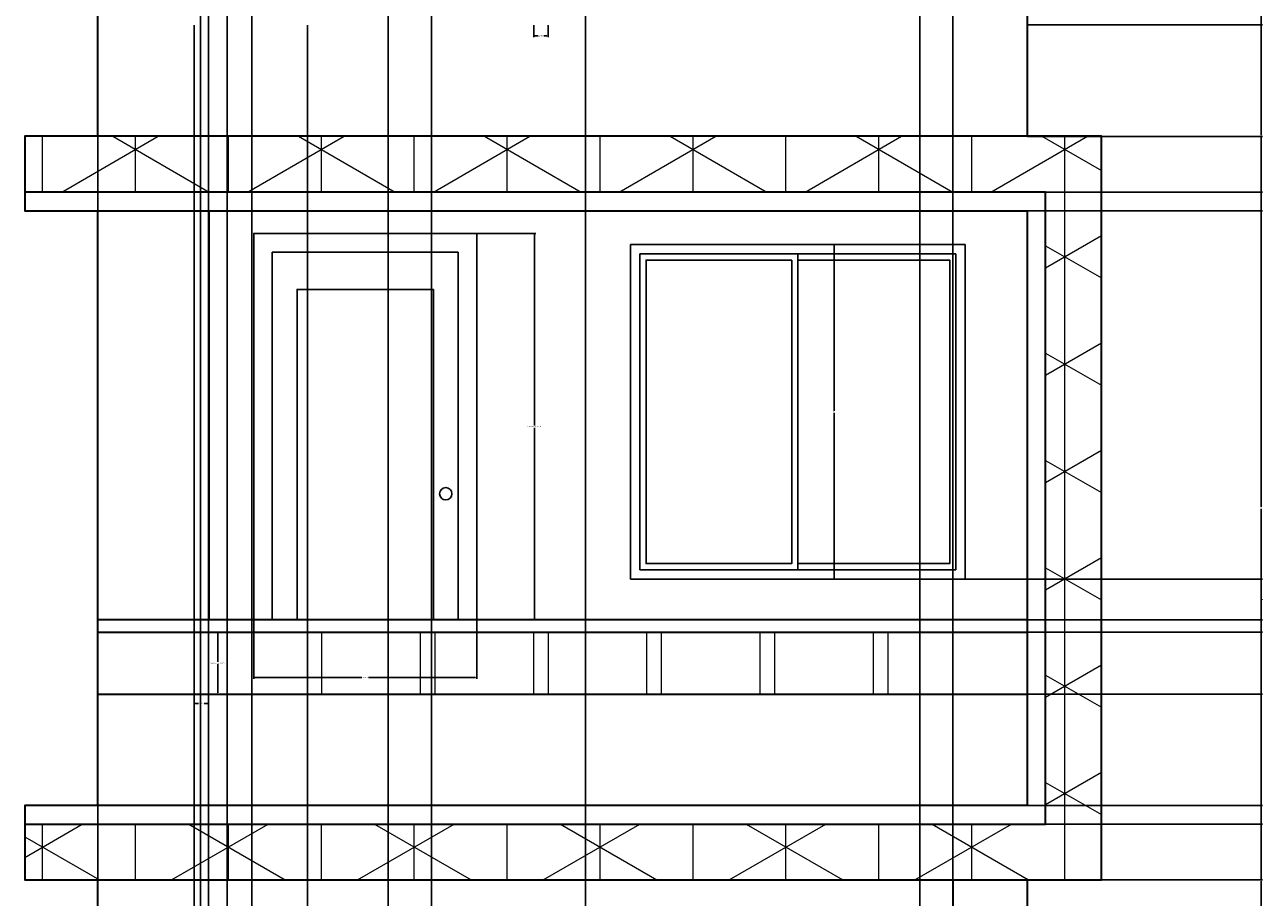
# Model space of a CAD drawing. Units: inches. Extents: x -3 to 302, y -138 to 325.
# Tile 3 of 5: x 102 to 302, y 1 to 141. Entities that reach past the tile are written whole.
import ezdxf

# ---------------------------------------------------------------- set-up
doc = ezdxf.new("R2010")
doc.units = ezdxf.units.IN
doc.header["$MEASUREMENT"] = 0
for name, color, linetype, lineweight in [('A-ANNO-DIMS', 2, 'Continuous', 18), ('A-DOOR', 4, 'Continuous', 25), ('A-ELEV', 7, 'Continuous', 35), ('A-ELEV-PATT', 8, 'Continuous', 13), ('A-ELEV-RAIL', 9, 'Continuous', 18), ('A-GLAZ', 3, 'Continuous', 25)]:
    doc.layers.add(name, color=color, linetype=linetype, lineweight=lineweight)
doc.styles.get("Standard").update_dxf_attribs({"font": 'arial.ttf'})
doc.dimstyles.get("Standard").update_dxf_attribs({"dimtxt": 0.18, "dimasz": 0.18, "dimexe": 0.18, "dimexo": 0.0625, "dimgap": 0.09, "dimtad": 0, "dimtih": 1, "dimtoh": 1, "dimdec": 4, "dimzin": 0, "dimdsep": 46, "dimtxsty": 'Standard', "dimcen": 0.09, "dimadec": 0, "dimazin": 0, "dimtfac": 1, "dimtdec": 4, "dimtofl": 0, "dimtmove": 0, "dimatfit": 3, "dimfxl": 1, "dimtolj": 1, "dimtzin": 0, "dimarcsym": 0})

# ---------------------------------------------------------------- blocks, each defined once
blk = doc.blocks.new('*U2')
for p, q in [((1.5, 1.5), (1.5, 52.5)), ((1.5, 52.5), (27, 52.5)), ((27, 1.5), (27, 52.5)), ((27, 52.5), (52.5, 52.5)), ((52.5, 52.5), (52.5, 1.5)), ((27, 1.5), (1.5, 1.5)), ((52.5, 1.5), (27, 1.5))]:
    blk.add_line(p, q)
blk.add_lwpolyline([(0, 0), (0, 54), (54, 54), (54, 0)], close=True)
for points in [[(26, 51.5), (26, 2.5), (2.5, 2.5), (2.5, 51.5), (26, 51.5)], [(27, 51.5), (51.5, 51.5), (51.5, 2.5), (27, 2.5)]]:
    blk.add_lwpolyline(points)
blk = doc.blocks.new('DOOR-FRAME-ELEV')
for points in [[(139.09, 45.37), (139.09, 107.7), (175.09, 107.7), (175.09, 45.37)], [(142.09, 45.37), (142.09, 104.67), (172.09, 104.67), (172.09, 45.37)], [(168.09, 45.37), (168.09, 98.67), (146.09, 98.67), (146.09, 45.37)]]:
    blk.add_lwpolyline(points)
blk = doc.blocks.new('RAIL-POST')
blk.add_lwpolyline([(239.12, 43.37), (241.43, 43.37), (241.43, 33.37), (239.12, 33.37)], close=True)
blk = doc.blocks.new('*D9')
at = {"layer": 'A-ANNO-DIMS', "color": 0, "lineweight": -2, "transparency": 16777216}
for p, q in [((175.15, 107.7), (184.61, 107.7)), ((184.43, 107.52), (184.43, 76.72)), ((184.43, 45.55), (184.43, 76.35)), ((175.15, 45.37), (184.61, 45.37))]:
    blk.add_line(p, q, dxfattribs=at)
at = {"layer": 'A-ANNO-DIMS', "color": 0, "transparency": 16777216}
for points in [[(184.4, 107.52), (184.46, 107.52), (184.43, 107.7)], [(184.4, 45.55), (184.46, 45.55), (184.43, 45.37)]]:
    blk.add_solid(points, dxfattribs=at)
at = {"layer": 'Defpoints', "color": 0, "transparency": 16777216}
for p in [(175.09, 107.7), (184.43, 107.7), (175.09, 45.37)]:
    blk.add_point(p, dxfattribs=at)
at = {"layer": 'A-ANNO-DIMS', "color": 0, "transparency": 16777216, "insert": (184.43, 76.54), "char_height": 0.18, "attachment_point": 5}
blk.add_mtext('\\A1;DOOR FRAME 62 TYP.', dxfattribs=at)
blk = doc.blocks.new('*D10')
at = {"layer": 'A-ANNO-DIMS', "color": 0, "lineweight": -2, "transparency": 16777216}
for p, q in [((139.09, 45.31), (139.09, 35.85)), ((175.09, 45.31), (175.09, 35.85)), ((139.27, 36.03), (156.56, 36.03)), ((174.91, 36.03), (157.61, 36.03))]:
    blk.add_line(p, q, dxfattribs=at)
at = {"layer": 'A-ANNO-DIMS', "color": 0, "transparency": 16777216}
for points in [[(139.27, 36.06), (139.27, 36), (139.09, 36.03)], [(174.91, 36.06), (174.91, 36), (175.09, 36.03)]]:
    blk.add_solid(points, dxfattribs=at)
at = {"layer": 'Defpoints', "color": 0, "transparency": 16777216}
for p in [(139.09, 45.37), (175.09, 45.37), (175.09, 36.03)]:
    blk.add_point(p, dxfattribs=at)
at = {"layer": 'A-ANNO-DIMS', "color": 0, "transparency": 16777216, "insert": (157.09, 36.03), "char_height": 0.18, "attachment_point": 5}
blk.add_mtext('\\A1;36 TYP.', dxfattribs=at)
blk = doc.blocks.new('*D13')
at = {"layer": 'A-ANNO-DIMS', "color": 0, "lineweight": -2, "transparency": 16777216}
for p, q in [((131.85, 43.37), (133.47, 43.37)), ((133.29, 43.19), (133.29, 38.56)), ((133.29, 33.55), (133.29, 38.19)), ((131.85, 33.37), (133.47, 33.37))]:
    blk.add_line(p, q, dxfattribs=at)
at = {"layer": 'A-ANNO-DIMS', "color": 0, "transparency": 16777216}
for points in [[(133.26, 43.19), (133.32, 43.19), (133.29, 43.37)], [(133.26, 33.55), (133.32, 33.55), (133.29, 33.37)]]:
    blk.add_solid(points, dxfattribs=at)
at = {"layer": 'Defpoints', "color": 0, "transparency": 16777216}
for p in [(131.79, 43.37), (133.29, 43.37), (131.79, 33.37)]:
    blk.add_point(p, dxfattribs=at)
at = {"layer": 'A-ANNO-DIMS', "color": 0, "transparency": 16777216, "insert": (133.29, 38.37), "char_height": 0.18, "attachment_point": 5}
blk.add_mtext('\\A1;RAILING POST 10 TYP.', dxfattribs=at)
blk = doc.blocks.new('*D14')
at = {"layer": 'A-ANNO-DIMS', "color": 0, "lineweight": -2, "transparency": 16777216}
for p, q in [((129.47, 33.31), (129.47, 31.69)), ((131.79, 33.31), (131.79, 31.69)), ((129.65, 31.87), (130.17, 31.87)), ((131.61, 31.87), (131.09, 31.87))]:
    blk.add_line(p, q, dxfattribs=at)
at = {"layer": 'A-ANNO-DIMS', "color": 0, "transparency": 16777216}
for points in [[(129.65, 31.9), (129.65, 31.84), (129.47, 31.87)], [(131.61, 31.9), (131.61, 31.84), (131.79, 31.87)]]:
    blk.add_solid(points, dxfattribs=at)
at = {"layer": 'Defpoints', "color": 0, "transparency": 16777216}
for p in [(129.47, 33.37), (131.79, 33.37), (131.79, 31.87)]:
    blk.add_point(p, dxfattribs=at)
at = {"layer": 'A-ANNO-DIMS', "color": 0, "transparency": 16777216, "insert": (130.63, 31.87), "char_height": 0.18, "attachment_point": 5}
blk.add_mtext('\\A1;2 TYP.', dxfattribs=at)
blk = doc.blocks.new('*D16')
at = {"layer": 'A-ANNO-DIMS', "color": 0, "lineweight": -2, "transparency": 16777216}
for p, q in [((184.3, 141.31), (184.3, 139.39)), ((186.61, 141.31), (186.61, 139.39)), ((184.48, 139.57), (184.99, 139.57)), ((186.43, 139.57), (185.91, 139.57))]:
    blk.add_line(p, q, dxfattribs=at)
at = {"layer": 'A-ANNO-DIMS', "color": 0, "transparency": 16777216}
for points in [[(184.48, 139.6), (184.48, 139.54), (184.3, 139.57)], [(186.43, 139.6), (186.43, 139.54), (186.61, 139.57)]]:
    blk.add_solid(points, dxfattribs=at)
at = {"layer": 'Defpoints', "color": 0, "transparency": 16777216}
for p in [(184.3, 141.37), (186.61, 141.37), (186.61, 139.57)]:
    blk.add_point(p, dxfattribs=at)
at = {"layer": 'A-ANNO-DIMS', "color": 0, "transparency": 16777216, "insert": (185.45, 139.57), "char_height": 0.18, "attachment_point": 5}
blk.add_mtext('\\A1;2 TYP.', dxfattribs=at)
blk = doc.blocks.new('*D19')
at = {"layer": 'A-ANNO-DIMS', "color": 0, "lineweight": -2, "transparency": 16777216}
for p, q in [((275.98, 3.37), (301.92, 3.37)), ((301.74, 3.19), (301.74, -56.44)), ((301.74, -116.45), (301.74, -56.81)), ((280.66, -116.63), (301.92, -116.63))]:
    blk.add_line(p, q, dxfattribs=at)
at = {"layer": 'A-ANNO-DIMS', "color": 0, "transparency": 16777216}
for points in [[(301.71, 3.19), (301.77, 3.19), (301.74, 3.37)], [(301.71, -116.45), (301.77, -116.45), (301.74, -116.63)]]:
    blk.add_solid(points, dxfattribs=at)
at = {"layer": 'Defpoints', "color": 0, "transparency": 16777216}
for p in [(275.92, 3.37), (301.74, 3.37), (280.59, -116.63)]:
    blk.add_point(p, dxfattribs=at)
at = {"layer": 'A-ANNO-DIMS', "color": 0, "transparency": 16777216, "insert": (301.74, -56.63), "char_height": 0.18, "attachment_point": 5}
blk.add_mtext('\\A1;120', dxfattribs=at)
blk = doc.blocks.new('*D20')
at = {"layer": 'A-ANNO-DIMS', "color": 0, "lineweight": -2, "transparency": 16777216}
for p, q in [((275.98, 123.37), (301.92, 123.37)), ((301.74, 123.19), (301.74, 63.56)), ((301.74, 3.55), (301.74, 63.19)), ((275.98, 3.37), (301.92, 3.37))]:
    blk.add_line(p, q, dxfattribs=at)
at = {"layer": 'A-ANNO-DIMS', "color": 0, "transparency": 16777216}
for points in [[(301.71, 123.19), (301.77, 123.19), (301.74, 123.37)], [(301.71, 3.55), (301.77, 3.55), (301.74, 3.37)]]:
    blk.add_solid(points, dxfattribs=at)
at = {"layer": 'Defpoints', "color": 0, "transparency": 16777216}
for p in [(275.92, 123.37), (301.74, 123.37), (275.92, 3.37)]:
    blk.add_point(p, dxfattribs=at)
at = {"layer": 'A-ANNO-DIMS', "color": 0, "transparency": 16777216, "insert": (301.74, 63.37), "char_height": 0.18, "attachment_point": 5}
blk.add_mtext('\\A1;120', dxfattribs=at)
blk = doc.blocks.new('*D21')
at = {"layer": 'A-ANNO-DIMS', "color": 0, "lineweight": -2, "transparency": 16777216}
for p, q in [((275.98, 243.37), (301.92, 243.37)), ((301.74, 243.19), (301.74, 183.56)), ((301.74, 123.55), (301.74, 183.19)), ((275.98, 123.37), (301.92, 123.37))]:
    blk.add_line(p, q, dxfattribs=at)
at = {"layer": 'A-ANNO-DIMS', "color": 0, "transparency": 16777216}
for points in [[(301.71, 243.19), (301.77, 243.19), (301.74, 243.37)], [(301.71, 123.55), (301.77, 123.55), (301.74, 123.37)]]:
    blk.add_solid(points, dxfattribs=at)
at = {"layer": 'Defpoints', "color": 0, "transparency": 16777216}
for p in [(275.92, 243.37), (301.74, 243.37), (275.92, 123.37)]:
    blk.add_point(p, dxfattribs=at)
at = {"layer": 'A-ANNO-DIMS', "color": 0, "transparency": 16777216, "insert": (301.74, 183.37), "char_height": 0.18, "attachment_point": 5}
blk.add_mtext('\\A1;120', dxfattribs=at)
blk = doc.blocks.new('*D40')
at = {"layer": 'A-ANNO-DIMS', "color": 0, "lineweight": -2, "transparency": 16777216}
for p, q in [((275.98, 123.37), (301.92, 123.37)), ((301.74, 123.19), (301.74, 119.06)), ((301.74, 114.55), (301.74, 118.69)), ((266.98, 114.37), (301.92, 114.37))]:
    blk.add_line(p, q, dxfattribs=at)
at = {"layer": 'A-ANNO-DIMS', "color": 0, "transparency": 16777216}
for points in [[(301.71, 123.19), (301.77, 123.19), (301.74, 123.37)], [(301.71, 114.55), (301.77, 114.55), (301.74, 114.37)]]:
    blk.add_solid(points, dxfattribs=at)
at = {"layer": 'Defpoints', "color": 0, "transparency": 16777216}
for p in [(275.92, 123.37), (266.92, 114.37), (301.74, 114.37)]:
    blk.add_point(p, dxfattribs=at)
at = {"layer": 'A-ANNO-DIMS', "color": 0, "transparency": 16777216, "insert": (301.74, 118.87), "char_height": 0.18, "attachment_point": 5}
blk.add_mtext('\\A1;9', dxfattribs=at)
blk = doc.blocks.new('*D41')
at = {"layer": 'A-ANNO-DIMS', "color": 0, "lineweight": -2, "transparency": 16777216}
for p, q in [((266.98, 114.37), (301.92, 114.37)), ((301.74, 114.19), (301.74, 113.06)), ((301.74, 111.55), (301.74, 112.69)), ((263.98, 111.37), (301.92, 111.37))]:
    blk.add_line(p, q, dxfattribs=at)
at = {"layer": 'A-ANNO-DIMS', "color": 0, "transparency": 16777216}
for points in [[(301.71, 114.19), (301.77, 114.19), (301.74, 114.37)], [(301.71, 111.55), (301.77, 111.55), (301.74, 111.37)]]:
    blk.add_solid(points, dxfattribs=at)
at = {"layer": 'Defpoints', "color": 0, "transparency": 16777216}
for p in [(266.92, 114.37), (263.92, 111.37), (301.74, 111.37)]:
    blk.add_point(p, dxfattribs=at)
at = {"layer": 'A-ANNO-DIMS', "color": 0, "transparency": 16777216, "insert": (301.74, 112.87), "char_height": 0.18, "attachment_point": 5}
blk.add_mtext('\\A1;3', dxfattribs=at)
blk = doc.blocks.new('*D42')
at = {"layer": 'A-ANNO-DIMS', "color": 0, "lineweight": -2, "transparency": 16777216}
for p, q in [((266.98, 12.37), (301.92, 12.37)), ((301.74, 12.19), (301.74, 8.06)), ((301.74, 3.55), (301.74, 7.69)), ((275.98, 3.37), (301.92, 3.37))]:
    blk.add_line(p, q, dxfattribs=at)
at = {"layer": 'A-ANNO-DIMS', "color": 0, "transparency": 16777216}
for points in [[(301.71, 12.19), (301.77, 12.19), (301.74, 12.37)], [(301.71, 3.55), (301.77, 3.55), (301.74, 3.37)]]:
    blk.add_solid(points, dxfattribs=at)
at = {"layer": 'Defpoints', "color": 0, "transparency": 16777216}
for p in [(266.92, 12.37), (301.74, 12.37), (275.92, 3.37)]:
    blk.add_point(p, dxfattribs=at)
at = {"layer": 'A-ANNO-DIMS', "color": 0, "transparency": 16777216, "insert": (301.74, 7.87), "char_height": 0.18, "attachment_point": 5}
blk.add_mtext('\\A1;9', dxfattribs=at)
blk = doc.blocks.new('*D43')
at = {"layer": 'A-ANNO-DIMS', "color": 0, "lineweight": -2, "transparency": 16777216}
for p, q in [((263.98, 15.37), (301.92, 15.37)), ((301.74, 15.19), (301.74, 14.06)), ((266.98, 12.37), (301.92, 12.37)), ((301.74, 12.55), (301.74, 13.69))]:
    blk.add_line(p, q, dxfattribs=at)
at = {"layer": 'A-ANNO-DIMS', "color": 0, "transparency": 16777216}
for points in [[(301.71, 15.19), (301.77, 15.19), (301.74, 15.37)], [(301.71, 12.55), (301.77, 12.55), (301.74, 12.37)]]:
    blk.add_solid(points, dxfattribs=at)
at = {"layer": 'Defpoints', "color": 0, "transparency": 16777216}
for p in [(263.92, 15.37), (301.74, 15.37), (266.92, 12.37)]:
    blk.add_point(p, dxfattribs=at)
at = {"layer": 'A-ANNO-DIMS', "color": 0, "transparency": 16777216, "insert": (301.74, 13.87), "char_height": 0.18, "attachment_point": 5}
blk.add_mtext('\\A1;3', dxfattribs=at)
blk = doc.blocks.new('*D44')
at = {"layer": 'A-ANNO-DIMS', "color": 0, "lineweight": -2, "transparency": 16777216}
for p, q in [((263.98, 33.37), (301.92, 33.37)), ((301.74, 33.19), (301.74, 24.56)), ((301.74, 15.55), (301.74, 24.19)), ((263.98, 15.37), (301.92, 15.37))]:
    blk.add_line(p, q, dxfattribs=at)
at = {"layer": 'A-ANNO-DIMS', "color": 0, "transparency": 16777216}
for points in [[(301.71, 33.19), (301.77, 33.19), (301.74, 33.37)], [(301.71, 15.55), (301.77, 15.55), (301.74, 15.37)]]:
    blk.add_solid(points, dxfattribs=at)
at = {"layer": 'Defpoints', "color": 0, "transparency": 16777216}
for p in [(263.92, 33.37), (301.74, 33.37), (263.92, 15.37)]:
    blk.add_point(p, dxfattribs=at)
at = {"layer": 'A-ANNO-DIMS', "color": 0, "transparency": 16777216, "insert": (301.74, 24.37), "char_height": 0.18, "attachment_point": 5}
blk.add_mtext('\\A1;18', dxfattribs=at)
blk = doc.blocks.new('*D45')
at = {"layer": 'A-ANNO-DIMS', "color": 0, "lineweight": -2, "transparency": 16777216}
for p, q in [((263.98, 43.37), (301.92, 43.37)), ((301.74, 43.19), (301.74, 38.56)), ((301.74, 33.55), (301.74, 38.19)), ((263.98, 33.37), (301.92, 33.37))]:
    blk.add_line(p, q, dxfattribs=at)
at = {"layer": 'A-ANNO-DIMS', "color": 0, "transparency": 16777216}
for points in [[(301.71, 43.19), (301.77, 43.19), (301.74, 43.37)], [(301.71, 33.55), (301.77, 33.55), (301.74, 33.37)]]:
    blk.add_solid(points, dxfattribs=at)
at = {"layer": 'Defpoints', "color": 0, "transparency": 16777216}
for p in [(263.92, 43.37), (301.74, 43.37), (263.92, 33.37)]:
    blk.add_point(p, dxfattribs=at)
at = {"layer": 'A-ANNO-DIMS', "color": 0, "transparency": 16777216, "insert": (301.74, 38.37), "char_height": 0.18, "attachment_point": 5}
blk.add_mtext('\\A1;10', dxfattribs=at)
blk = doc.blocks.new('*D46')
at = {"layer": 'A-ANNO-DIMS', "color": 0, "lineweight": -2, "transparency": 16777216}
for p, q in [((263.98, 45.37), (301.92, 45.37)), ((301.74, 45.19), (301.74, 44.56)), ((301.74, 43.55), (301.74, 44.19)), ((263.98, 43.37), (301.92, 43.37))]:
    blk.add_line(p, q, dxfattribs=at)
at = {"layer": 'A-ANNO-DIMS', "color": 0, "transparency": 16777216}
for points in [[(301.71, 45.19), (301.77, 45.19), (301.74, 45.37)], [(301.71, 43.55), (301.77, 43.55), (301.74, 43.37)]]:
    blk.add_solid(points, dxfattribs=at)
at = {"layer": 'Defpoints', "color": 0, "transparency": 16777216}
for p in [(263.92, 45.37), (301.74, 45.37), (263.92, 43.37)]:
    blk.add_point(p, dxfattribs=at)
at = {"layer": 'A-ANNO-DIMS', "color": 0, "transparency": 16777216, "insert": (301.74, 44.37), "char_height": 0.18, "attachment_point": 5}
blk.add_mtext('\\A1;2', dxfattribs=at)
blk = doc.blocks.new('*D47')
at = {"layer": 'A-ANNO-DIMS', "color": 0, "lineweight": -2, "transparency": 16777216}
for p, q in [((254, 51.91), (301.92, 51.91)), ((301.74, 51.73), (301.74, 48.83)), ((301.74, 45.55), (301.74, 48.46)), ((263.98, 45.37), (301.92, 45.37))]:
    blk.add_line(p, q, dxfattribs=at)
at = {"layer": 'A-ANNO-DIMS', "color": 0, "transparency": 16777216}
for points in [[(301.71, 51.73), (301.77, 51.73), (301.74, 51.91)], [(301.71, 45.55), (301.77, 45.55), (301.74, 45.37)]]:
    blk.add_solid(points, dxfattribs=at)
at = {"layer": 'Defpoints', "color": 0, "transparency": 16777216}
for p in [(253.94, 51.91), (301.74, 51.91), (263.92, 45.37)]:
    blk.add_point(p, dxfattribs=at)
at = {"layer": 'A-ANNO-DIMS', "color": 0, "transparency": 16777216, "insert": (301.74, 48.64), "char_height": 0.18, "attachment_point": 5}
blk.add_mtext('\\A1;6.539', dxfattribs=at)
blk = doc.blocks.new('*D48')
at = {"layer": 'A-ANNO-DIMS', "color": 0, "lineweight": -2, "transparency": 16777216}
for p, q in [((253.87, 105.91), (232.61, 105.91)), ((232.79, 105.73), (232.79, 79.1)), ((232.79, 52.09), (232.79, 78.73)), ((253.87, 51.91), (232.61, 51.91))]:
    blk.add_line(p, q, dxfattribs=at)
at = {"layer": 'A-ANNO-DIMS', "color": 0, "transparency": 16777216}
for points in [[(232.76, 105.73), (232.82, 105.73), (232.79, 105.91)], [(232.76, 52.09), (232.82, 52.09), (232.79, 51.91)]]:
    blk.add_solid(points, dxfattribs=at)
at = {"layer": 'Defpoints', "color": 0, "transparency": 16777216}
for p in [(232.79, 105.91), (253.94, 105.91), (253.94, 51.91)]:
    blk.add_point(p, dxfattribs=at)
at = {"layer": 'A-ANNO-DIMS', "color": 0, "transparency": 16777216, "insert": (232.79, 78.91), "char_height": 0.18, "attachment_point": 5}
blk.add_mtext('\\A1;54', dxfattribs=at)
blk = doc.blocks.new('*D49')
at = {"layer": 'A-ANNO-DIMS', "color": 0, "lineweight": -2, "transparency": 16777216}
for p, q in [((263.98, 141.37), (301.92, 141.37)), ((301.74, 141.19), (301.74, 132.56)), ((301.74, 123.55), (301.74, 132.19)), ((263.98, 123.37), (301.92, 123.37))]:
    blk.add_line(p, q, dxfattribs=at)
at = {"layer": 'A-ANNO-DIMS', "color": 0, "transparency": 16777216}
for points in [[(301.71, 141.19), (301.77, 141.19), (301.74, 141.37)], [(301.71, 123.55), (301.77, 123.55), (301.74, 123.37)]]:
    blk.add_solid(points, dxfattribs=at)
at = {"layer": 'Defpoints', "color": 0, "transparency": 16777216}
for p in [(263.92, 141.37), (301.74, 141.37), (263.92, 123.37)]:
    blk.add_point(p, dxfattribs=at)
at = {"layer": 'A-ANNO-DIMS', "color": 0, "transparency": 16777216, "insert": (301.74, 132.37), "char_height": 0.18, "attachment_point": 5}
blk.add_mtext('\\A1;18', dxfattribs=at)
blk = doc.blocks.new('*D66')
at = {"layer": 'A-ANNO-DIMS', "color": 0, "lineweight": -2, "transparency": 16777216}
for p, q in [((113.92, 141.31), (113.92, -137.96)), ((129.47, 141.31), (129.47, -137.96)), ((114.1, -137.78), (121.24, -137.78)), ((129.29, -137.78), (122.15, -137.78))]:
    blk.add_line(p, q, dxfattribs=at)
at = {"layer": 'A-ANNO-DIMS', "color": 0, "transparency": 16777216}
for points in [[(114.1, -137.75), (114.1, -137.81), (113.92, -137.78)], [(129.29, -137.75), (129.29, -137.81), (129.47, -137.78)]]:
    blk.add_solid(points, dxfattribs=at)
at = {"layer": 'Defpoints', "color": 0, "transparency": 16777216}
for p in [(113.92, 141.37), (129.47, 141.37), (129.47, -137.78)]:
    blk.add_point(p, dxfattribs=at)
at = {"layer": 'A-ANNO-DIMS', "color": 0, "transparency": 16777216, "insert": (121.7, -137.78), "char_height": 0.18, "attachment_point": 5}
blk.add_mtext('\\A1;15.553', dxfattribs=at)
blk = doc.blocks.new('*D67')
at = {"layer": 'A-ANNO-DIMS', "color": 0, "lineweight": -2, "transparency": 16777216}
for p, q in [((129.47, 141.31), (129.47, -137.96)), ((147.75, 141.31), (147.75, -137.96)), ((129.65, -137.78), (138.16, -137.78)), ((147.57, -137.78), (139.07, -137.78))]:
    blk.add_line(p, q, dxfattribs=at)
at = {"layer": 'A-ANNO-DIMS', "color": 0, "transparency": 16777216}
for points in [[(129.65, -137.75), (129.65, -137.81), (129.47, -137.78)], [(147.57, -137.75), (147.57, -137.81), (147.75, -137.78)]]:
    blk.add_solid(points, dxfattribs=at)
at = {"layer": 'Defpoints', "color": 0, "transparency": 16777216}
for p in [(129.47, 141.37), (147.75, 141.37), (147.75, -137.78)]:
    blk.add_point(p, dxfattribs=at)
at = {"layer": 'A-ANNO-DIMS', "color": 0, "transparency": 16777216, "insert": (138.61, -137.78), "char_height": 0.18, "attachment_point": 5}
blk.add_mtext('\\A1;18.274', dxfattribs=at)
blk = doc.blocks.new('*D68')
at = {"layer": 'A-ANNO-DIMS', "color": 0, "lineweight": -2, "transparency": 16777216}
for p, q in [((130.489456, -43.793388), (130.489456, 324.704711)), ((130.669456, 324.524711), (130.823276, 324.524711)), ((131.607096, 324.524711), (131.453276, 324.524711)), ((131.787096, -26.240874), (131.787096, 324.704711))]:
    blk.add_line(p, q, dxfattribs=at)
at = {"layer": 'A-ANNO-DIMS', "color": 0, "transparency": 16777216}
for points in [[(130.669456, 324.554711), (130.669456, 324.494711), (130.489456, 324.524711)], [(131.607096, 324.554711), (131.607096, 324.494711), (131.787096, 324.524711)]]:
    blk.add_solid(points, dxfattribs=at)
at = {"layer": 'Defpoints', "color": 0, "transparency": 16777216}
for p in [(131.787096, 324.524711), (131.787096, -26.303374), (130.489456, -43.855888)]:
    blk.add_point(p, dxfattribs=at)
at = {"layer": 'A-ANNO-DIMS', "color": 0, "transparency": 16777216, "insert": (131.138276, 324.524711), "char_height": 0.18, "attachment_point": 5}
blk.add_mtext('\\A1;1.30', dxfattribs=at)
blk = doc.blocks.new('*D69')
at = {"layer": 'A-ANNO-DIMS', "color": 0, "lineweight": -2, "transparency": 16777216}
for p, q in [((131.79, -26.24), (131.79, 324.7)), ((131.97, 324.52), (149.57, 324.52)), ((167.61, 324.52), (150.01, 324.52)), ((167.79, -26.24), (167.79, 324.7))]:
    blk.add_line(p, q, dxfattribs=at)
at = {"layer": 'A-ANNO-DIMS', "color": 0, "transparency": 16777216}
for points in [[(131.97, 324.55), (131.97, 324.49), (131.79, 324.52)], [(167.61, 324.55), (167.61, 324.49), (167.79, 324.52)]]:
    blk.add_solid(points, dxfattribs=at)
at = {"layer": 'Defpoints', "color": 0, "transparency": 16777216}
for p in [(167.79, 324.52), (131.79, -26.3), (167.79, -26.3)]:
    blk.add_point(p, dxfattribs=at)
at = {"layer": 'A-ANNO-DIMS', "color": 0, "transparency": 16777216, "insert": (149.79, 324.52), "char_height": 0.18, "attachment_point": 5}
blk.add_mtext('\\A1;36', dxfattribs=at)
blk = doc.blocks.new('*D70')
at = {"layer": 'A-ANNO-DIMS', "color": 0, "lineweight": -2, "transparency": 16777216}
for p, q in [((167.79, -26.24), (167.79, 324.7)), ((167.97, 324.52), (179.82, 324.52)), ((192.46, 324.52), (180.61, 324.52)), ((192.64, -28.02), (192.64, 324.7))]:
    blk.add_line(p, q, dxfattribs=at)
at = {"layer": 'A-ANNO-DIMS', "color": 0, "transparency": 16777216}
for points in [[(167.97, 324.55), (167.97, 324.49), (167.79, 324.52)], [(192.46, 324.55), (192.46, 324.49), (192.64, 324.52)]]:
    blk.add_solid(points, dxfattribs=at)
at = {"layer": 'Defpoints', "color": 0, "transparency": 16777216}
for p in [(192.64, 324.52), (167.79, -26.3), (192.64, -28.09)]:
    blk.add_point(p, dxfattribs=at)
at = {"layer": 'A-ANNO-DIMS', "color": 0, "transparency": 16777216, "insert": (180.21, 324.52), "char_height": 0.18, "attachment_point": 5}
blk.add_mtext('\\A1;24.85', dxfattribs=at)
blk = doc.blocks.new('*D71')
at = {"layer": 'A-ANNO-DIMS', "color": 0, "lineweight": -2, "transparency": 16777216}
for p, q in [((192.64, -28.02), (192.64, 324.7)), ((192.82, 324.52), (219.42, 324.52)), ((246.46, 324.52), (219.86, 324.52)), ((246.64, -28.02), (246.64, 324.7))]:
    blk.add_line(p, q, dxfattribs=at)
at = {"layer": 'A-ANNO-DIMS', "color": 0, "transparency": 16777216}
for points in [[(192.82, 324.55), (192.82, 324.49), (192.64, 324.52)], [(246.46, 324.55), (246.46, 324.49), (246.64, 324.52)]]:
    blk.add_solid(points, dxfattribs=at)
at = {"layer": 'Defpoints', "color": 0, "transparency": 16777216}
for p in [(246.64, 324.52), (192.64, -28.09), (246.64, -28.09)]:
    blk.add_point(p, dxfattribs=at)
at = {"layer": 'A-ANNO-DIMS', "color": 0, "transparency": 16777216, "insert": (219.64, 324.52), "char_height": 0.18, "attachment_point": 5}
blk.add_mtext('\\A1;54', dxfattribs=at)
blk = doc.blocks.new('*D72')
at = {"layer": 'A-ANNO-DIMS', "color": 0, "lineweight": -2, "transparency": 16777216}
for p, q in [((246.64, -28.02), (246.64, 324.7)), ((246.82, 324.52), (248.89, 324.52)), ((251.74, 324.52), (249.67, 324.52)), ((251.92, -49.03), (251.92, 324.7))]:
    blk.add_line(p, q, dxfattribs=at)
at = {"layer": 'A-ANNO-DIMS', "color": 0, "transparency": 16777216}
for points in [[(246.82, 324.55), (246.82, 324.49), (246.64, 324.52)], [(251.74, 324.55), (251.74, 324.49), (251.92, 324.52)]]:
    blk.add_solid(points, dxfattribs=at)
at = {"layer": 'Defpoints', "color": 0, "transparency": 16777216}
for p in [(251.92, 324.52), (246.64, -28.09), (251.92, -49.09)]:
    blk.add_point(p, dxfattribs=at)
at = {"layer": 'A-ANNO-DIMS', "color": 0, "transparency": 16777216, "insert": (249.28, 324.52), "char_height": 0.18, "attachment_point": 5}
blk.add_mtext('\\A1;5.285', dxfattribs=at)
blk = doc.blocks.new('*D73')
at = {"layer": 'A-ANNO-DIMS', "color": 0, "lineweight": -2, "transparency": 16777216}
for p, q in [((131.79, -26.24), (131.79, 324.7)), ((131.97, 324.52), (133.14, 324.52)), ((134.61, 324.52), (133.44, 324.52)), ((134.79, -29.26), (134.79, 324.7))]:
    blk.add_line(p, q, dxfattribs=at)
at = {"layer": 'A-ANNO-DIMS', "color": 0, "transparency": 16777216}
for points in [[(131.97, 324.55), (131.97, 324.49), (131.79, 324.52)], [(134.61, 324.55), (134.61, 324.49), (134.79, 324.52)]]:
    blk.add_solid(points, dxfattribs=at)
at = {"layer": 'Defpoints', "color": 0, "transparency": 16777216}
for p in [(134.79, 324.52), (131.79, -26.3), (134.79, -29.33)]:
    blk.add_point(p, dxfattribs=at)
at = {"layer": 'A-ANNO-DIMS', "color": 0, "transparency": 16777216, "insert": (133.29, 324.52), "char_height": 0.18, "attachment_point": 5}
blk.add_mtext('\\A1;3', dxfattribs=at)
blk = doc.blocks.new('*D74')
at = {"layer": 'A-ANNO-DIMS', "color": 0, "lineweight": -2, "transparency": 16777216}
for p, q in [((134.79, -29.26), (134.79, 324.7)), ((134.97, 324.52), (136.63, 324.52)), ((138.61, 324.52), (136.94, 324.52)), ((138.79, -35.26), (138.79, 324.7))]:
    blk.add_line(p, q, dxfattribs=at)
at = {"layer": 'A-ANNO-DIMS', "color": 0, "transparency": 16777216}
for points in [[(134.97, 324.55), (134.97, 324.49), (134.79, 324.52)], [(138.61, 324.55), (138.61, 324.49), (138.79, 324.52)]]:
    blk.add_solid(points, dxfattribs=at)
at = {"layer": 'Defpoints', "color": 0, "transparency": 16777216}
for p in [(138.79, 324.52), (134.79, -29.33), (138.79, -35.33)]:
    blk.add_point(p, dxfattribs=at)
at = {"layer": 'A-ANNO-DIMS', "color": 0, "transparency": 16777216, "insert": (136.79, 324.52), "char_height": 0.18, "attachment_point": 5}
blk.add_mtext('\\A1;4', dxfattribs=at)
blk = doc.blocks.new('*D75')
at = {"layer": 'A-ANNO-DIMS', "color": 0, "lineweight": -2, "transparency": 16777216}
for p, q in [((138.79, -35.26), (138.79, 324.7)), ((138.97, 324.52), (149.57, 324.52)), ((160.61, 324.52), (150.01, 324.52)), ((160.79, -35.26), (160.79, 324.7))]:
    blk.add_line(p, q, dxfattribs=at)
at = {"layer": 'A-ANNO-DIMS', "color": 0, "transparency": 16777216}
for points in [[(138.97, 324.55), (138.97, 324.49), (138.79, 324.52)], [(160.61, 324.55), (160.61, 324.49), (160.79, 324.52)]]:
    blk.add_solid(points, dxfattribs=at)
at = {"layer": 'Defpoints', "color": 0, "transparency": 16777216}
for p in [(160.79, 324.52), (138.79, -35.33), (160.79, -35.33)]:
    blk.add_point(p, dxfattribs=at)
at = {"layer": 'A-ANNO-DIMS', "color": 0, "transparency": 16777216, "insert": (149.79, 324.52), "char_height": 0.18, "attachment_point": 5}
blk.add_mtext('\\A1;22', dxfattribs=at)

msp = doc.modelspace()

# ---------------------------------------------------------------- hatches: boundary and pattern name
at = {"layer": 'A-ELEV-PATT'}
h = msp.add_hatch(dxfattribs=at)
h.set_pattern_fill('NET3', color=256, scale=120, angle=90)
h.paths.add_polyline_path([(275.922, 123.3747), (102.135, 123.3747), (102.135, 114.3747), (266.922, 114.3747), (266.922, 12.3747), (102.135, 12.3747), (102.135, 3.3747), (275.922, 3.3747)])
h.paths.add_polyline_path([(275.922, 243.3747), (263.922, 243.3747), (113.922, 243.3747), (102.135, 243.3747), (102.135, 231.3747), (113.922, 231.3747), (263.922, 231.3747), (275.922, 231.3747)])

# ---------------------------------------------------------------- linework, layer by layer
at = {"layer": 'A-DOOR'}
msp.add_circle((170.0861, 65.6966), 1, dxfattribs=at)
at = {"layer": 'A-ELEV'}
for p, q in [((113.922, 123.3747), (113.922, 231.3747)), ((263.922, 231.3747), (263.922, 123.3747)), ((263.922, 153.3747), (263.922, 123.3747)), ((113.922, 15.3747), (113.922, 111.3747)), ((131.922, 45.3747), (131.922, 111.3747)), ((113.922, 45.3747), (263.922, 45.3747)), ((113.922, 43.3747), (263.922, 43.3747)), ((113.922, 33.3747), (263.922, 33.3747)), ((113.922, -49.0923), (113.922, 3.3747)), ((251.922, 3.3747), (251.922, -116.6253)), ((263.922, 3.3747), (263.922, -49.0923))]:
    msp.add_line(p, q, dxfattribs=at)
for points in [[(113.922, 123.3747), (102.135, 123.3747), (102.135, 111.3747), (113.922, 111.3747), (263.922, 111.3747), (263.922, 15.3747), (113.922, 15.3747), (102.135, 15.3747), (102.135, 3.3747), (113.922, 3.3747)], [(102.135, 3.3747), (275.922, 3.3747), (275.922, 123.3747), (102.135, 123.3747)], [(102.135, 12.3747), (266.922, 12.3747), (266.922, 114.3747), (102.135, 114.3747)]]:
    msp.add_lwpolyline(points, dxfattribs=at)

# ---------------------------------------------------------------- block references
at = {"layer": 'A-DOOR'}
msp.add_blockref('DOOR-FRAME-ELEV', (0, 0), dxfattribs=at)
at = {"layer": 'A-ELEV-RAIL'}
for p in [(-109.6443, 0), (-91.3703, 0), (-73.0962, 0), (-54.8222, 0), (-36.5481, 0), (-18.2741, 0), (0, 0)]:
    msp.add_blockref('RAIL-POST', p, dxfattribs=at)
at = {"layer": 'A-GLAZ'}
msp.add_blockref('*U2', (199.9358, 51.9138), dxfattribs=at)

# ---------------------------------------------------------------- dimensions: what is measured, and where the dimension line sits
at = {"layer": 'A-ANNO-DIMS'}
for base, p1, p2, override, picture, middle in [((131.7871, 324.5247), (130.4895, -43.8559), (131.7871, -26.3034), {"dimdec": 2, "dimlfac": 1, "dimrnd": 0, "dimzin": 0, "dimdsep": 46, "dimlunit": 2}, '*D68', (131.1383, 324.5247)), ((167.7871, 324.5247), (131.7871, -26.3034), (167.7871, -26.3034), {"dimdec": 0, "dimlfac": 1, "dimrnd": 0, "dimzin": 0, "dimdsep": 46, "dimlunit": 2}, '*D69', (149.7871, 324.5247)), ((134.7871, 324.5247), (131.7871, -26.3034), (134.7871, -29.3264), {"dimdec": 0, "dimlfac": 1, "dimrnd": 0, "dimzin": 0, "dimdsep": 46, "dimlunit": 2}, '*D73', (133.2871, 324.5247)), ((138.7871, 324.5247), (134.7871, -29.3264), (138.7871, -35.3264), {"dimdec": 0, "dimlfac": 1, "dimrnd": 0, "dimzin": 0, "dimdsep": 46, "dimlunit": 2}, '*D74', (136.7871, 324.5247)), ((160.7871, 324.5247), (138.7871, -35.3264), (160.7871, -35.3264), {"dimdec": 0, "dimlfac": 1, "dimrnd": 0, "dimzin": 0, "dimdsep": 46, "dimlunit": 2}, '*D75', (149.7871, 324.5247)), ((192.6368, 324.5247), (167.7871, -26.3034), (192.6368, -28.0862), {"dimdec": 2, "dimlfac": 1, "dimrnd": 0, "dimzin": 0, "dimdsep": 46, "dimlunit": 2}, '*D70', (180.2119, 324.5247)), ((246.6368, 324.5247), (192.6368, -28.0862), (246.6368, -28.0862), {"dimdec": 0, "dimlfac": 1, "dimrnd": 0, "dimzin": 0, "dimdsep": 46, "dimlunit": 2}, '*D71', (219.6368, 324.5247)), ((251.922, 324.5247), (246.6368, -28.0862), (251.922, -49.0923), {"dimdec": 3, "dimlfac": 1, "dimrnd": 0, "dimzin": 0, "dimdsep": 46, "dimlunit": 2}, '*D72', (249.2794, 324.5247)), ((129.4748, -137.7753), (113.922, 141.3747), (129.4748, 141.3747), {"dimdec": 3, "dimlfac": 1, "dimrnd": 0, "dimzin": 0, "dimdsep": 46, "dimlunit": 2}, '*D66', (121.6984, -137.7753)), ((147.7489, -137.7753), (129.4748, 141.3747), (147.7489, 141.3747), {"dimdec": 3, "dimlfac": 1, "dimrnd": 0, "dimzin": 0, "dimdsep": 46, "dimlunit": 2}, '*D67', (138.6118, -137.7753))]:
    dim = msp.add_linear_dim(base=base, p1=p1, p2=p2, dimstyle='Standard', override=override, dxfattribs=at)
    dim.commit()
    dim.dimension.update_dxf_attribs({"geometry": picture, "text_midpoint": middle})
for base, p1, p2, override, picture, middle in [((301.7436, 243.3747), (275.922, 123.3747), (275.922, 243.3747), {"dimdec": 0, "dimlfac": 1, "dimrnd": 0, "dimzin": 0, "dimdsep": 46, "dimlunit": 2}, '*D21', (301.7436, 183.3747)), ((301.7436, 141.3747), (263.922, 123.3747), (263.922, 141.3747), {"dimdec": 0, "dimlfac": 1, "dimrnd": 0, "dimzin": 0, "dimdsep": 46, "dimlunit": 2}, '*D49', (301.7436, 132.3747)), ((301.7436, 114.3747), (275.922, 123.3747), (266.922, 114.3747), {"dimdec": 0, "dimlfac": 1, "dimrnd": 0, "dimzin": 0, "dimdsep": 46, "dimlunit": 2}, '*D40', (301.7436, 118.8747)), ((301.7436, 123.3747), (275.922, 3.3747), (275.922, 123.3747), {"dimdec": 0, "dimlfac": 1, "dimrnd": 0, "dimzin": 0, "dimdsep": 46, "dimlunit": 2}, '*D20', (301.7436, 63.3747)), ((301.7436, 111.3747), (266.922, 114.3747), (263.922, 111.3747), {"dimdec": 0, "dimlfac": 1, "dimrnd": 0, "dimzin": 0, "dimdsep": 46, "dimlunit": 2}, '*D41', (301.7436, 112.8747)), ((232.7858, 105.9138), (253.9358, 51.9138), (253.9358, 105.9138), {"dimdec": 0, "dimlfac": 1, "dimrnd": 0, "dimzin": 0, "dimdsep": 46, "dimlunit": 2}, '*D48', (232.7858, 78.9138)), ((301.7436, 51.9138), (263.922, 45.3747), (253.9358, 51.9138), {"dimdec": 3, "dimlfac": 1, "dimrnd": 0, "dimzin": 0, "dimdsep": 46, "dimlunit": 2}, '*D47', (301.7436, 48.6443)), ((301.7436, 45.3747), (263.922, 43.3747), (263.922, 45.3747), {"dimdec": 0, "dimlfac": 1, "dimrnd": 0, "dimzin": 0, "dimdsep": 46, "dimlunit": 2}, '*D46', (301.7436, 44.3747)), ((301.7436, 43.3747), (263.922, 33.3747), (263.922, 43.3747), {"dimdec": 0, "dimlfac": 1, "dimrnd": 0, "dimzin": 0, "dimdsep": 46, "dimlunit": 2}, '*D45', (301.7436, 38.3747)), ((301.7436, 33.3747), (263.922, 15.3747), (263.922, 33.3747), {"dimdec": 0, "dimlfac": 1, "dimrnd": 0, "dimzin": 0, "dimdsep": 46, "dimlunit": 2}, '*D44', (301.7436, 24.3747)), ((301.7436, 15.3747), (266.922, 12.3747), (263.922, 15.3747), {"dimdec": 0, "dimlfac": 1, "dimrnd": 0, "dimzin": 0, "dimdsep": 46, "dimlunit": 2}, '*D43', (301.7436, 13.8747)), ((301.7436, 12.3747), (275.922, 3.3747), (266.922, 12.3747), {"dimdec": 0, "dimlfac": 1, "dimrnd": 0, "dimzin": 0, "dimdsep": 46, "dimlunit": 2}, '*D42', (301.7436, 7.8747)), ((301.7436, 3.3747), (280.5936, -116.6253), (275.922, 3.3747), {"dimdec": 0, "dimlfac": 1, "dimrnd": 0, "dimzin": 0, "dimdsep": 46, "dimlunit": 2}, '*D19', (301.7436, -56.6253))]:
    dim = msp.add_linear_dim(base=base, p1=p1, p2=p2, angle=90, dimstyle='Standard', override=override, dxfattribs=at)
    dim.commit()
    dim.dimension.update_dxf_attribs({"geometry": picture, "text_midpoint": middle})
for base, p1, p2, picture, middle in [((186.6093, 139.5747), (184.297, 141.3747), (186.6093, 141.3747), '*D16', (185.4531, 139.5747)), ((175.0861, 36.0264), (139.0861, 45.3747), (175.0861, 45.3747), '*D10', (157.0861, 36.0264)), ((131.7871, 31.8747), (129.4748, 33.3747), (131.7871, 33.3747), '*D14', (130.631, 31.8747))]:
    dim = msp.add_linear_dim(base=base, p1=p1, p2=p2, text='<> TYP.', dimstyle='Standard', override={"dimdec": 0, "dimlfac": 1, "dimrnd": 0, "dimzin": 0, "dimdsep": 46, "dimlunit": 2}, dxfattribs=at)
    dim.commit()
    dim.dimension.update_dxf_attribs({"geometry": picture, "text_midpoint": middle})
for base, p1, p2, text, picture, middle in [((184.4344, 107.6966), (175.0861, 45.3747), (175.0861, 107.6966), 'DOOR FRAME <> TYP.', '*D9', (184.4344, 76.5357)), ((133.2871, 43.3747), (131.7871, 33.3747), (131.7871, 43.3747), 'RAILING POST <> TYP.', '*D13', (133.2871, 38.3747))]:
    dim = msp.add_linear_dim(base=base, p1=p1, p2=p2, angle=90, text=text, dimstyle='Standard', override={"dimdec": 0, "dimlfac": 1, "dimrnd": 0, "dimzin": 0, "dimdsep": 46, "dimlunit": 2}, dxfattribs=at)
    dim.commit()
    dim.dimension.update_dxf_attribs({"geometry": picture, "text_midpoint": middle})

doc.saveas('drawing.dxf')
